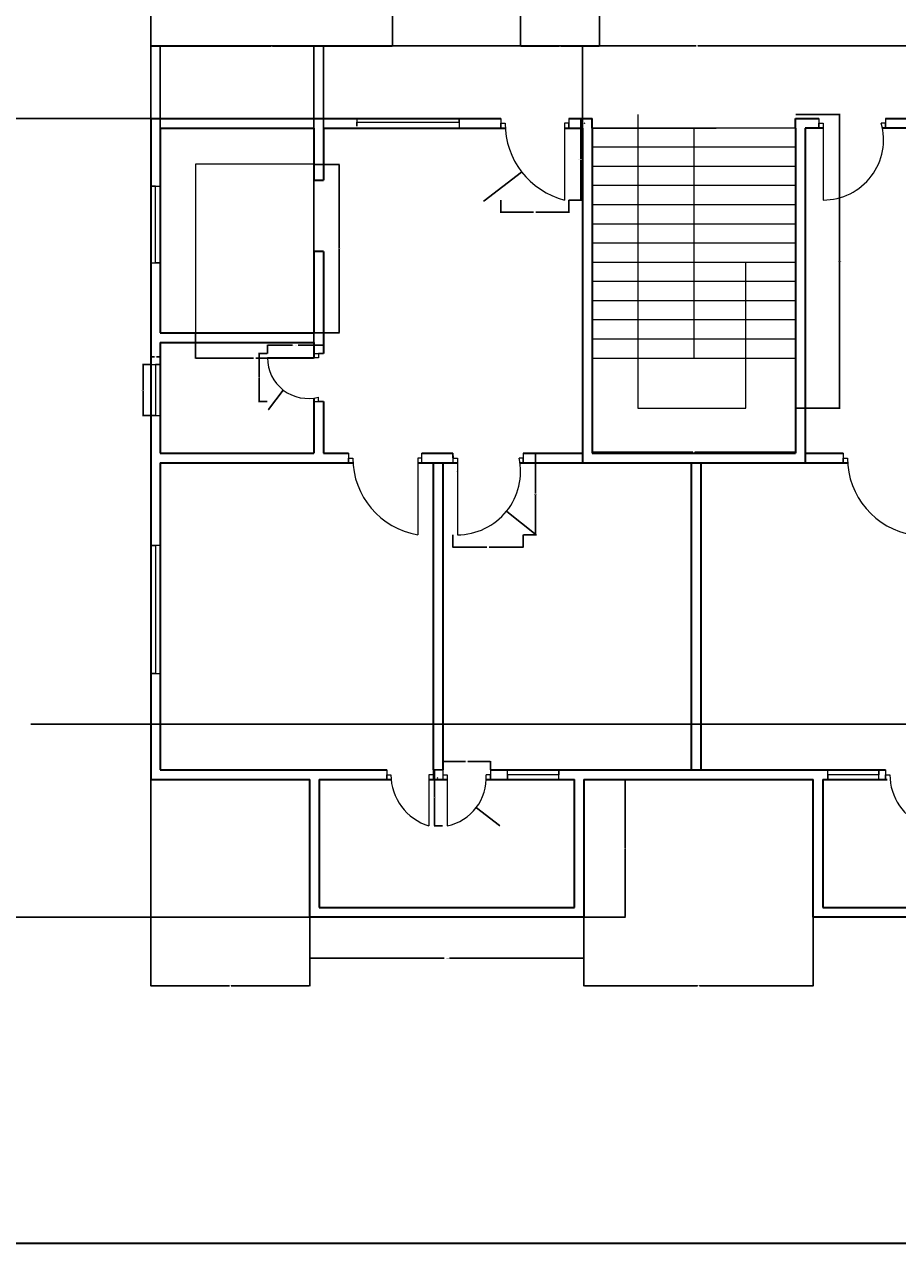
# Model space of a CAD drawing. Units: inches. Extents: x 2055 to 3558, y 1520 to 2888.
# Tile 5 of 8: x 2732 to 3142, y 1520 to 2092. Entities that reach past the tile are written whole.
import ezdxf

# ---------------------------------------------------------------- set-up
doc = ezdxf.new("R2010")
doc.units = ezdxf.units.IN
for name, color, linetype, lineweight in [('A-ANNO-DIMS', 2, 'Continuous', 18), ('A-ANNO-SYMB', 7, 'Continuous', 25), ('A-ANNO-TTLB', 7, 'Continuous', 35), ('A-DOOR', 3, 'Continuous', 18), ('A-FLOR-FIXT', 8, 'Continuous', 18), ('A-FLOR-STRS', 7, 'Continuous', 18), ('A-GLAZ', 4, 'Continuous', 18), ('A-WALL', 7, 'Continuous', 35)]:
    doc.layers.add(name, color=color, linetype=linetype, lineweight=lineweight)
doc.styles.get("Standard").update_dxf_attribs({"font": 'arial.ttf'})
doc.dimstyles.get("Standard").update_dxf_attribs({"dimtxt": 0.18, "dimasz": 0.18, "dimexe": 0.18, "dimexo": 0.0625, "dimgap": 0.09, "dimtad": 0, "dimtih": 1, "dimtoh": 1, "dimdec": 4, "dimzin": 0, "dimdsep": 46, "dimtxsty": 'Standard', "dimcen": 0.09, "dimadec": 0, "dimazin": 0, "dimtfac": 1, "dimtdec": 4, "dimtofl": 0, "dimtmove": 0, "dimatfit": 3, "dimfxl": 1, "dimtolj": 1, "dimtzin": 0, "dimarcsym": 0})

# ---------------------------------------------------------------- blocks, each defined once
blk = doc.blocks.new('DOOR-ENTRY-36-C')
for p, q in [((0, 38.25), (0, 33.75)), ((0, 33.75), (0, 36)), ((0, 36), (2, 36)), ((31.88, 36), (29.88, 36)), ((29.88, 36), (29.88, 0)), ((31.88, 38.25), (31.88, 33.75)), ((31.88, 33.75), (31.88, 36))]:
    blk.add_line(p, q)
blk.add_arc((39.18, 36), 37.18, 180, 255.5126)
blk = doc.blocks.new('DOOR-BATH-24-C')
for p, q in [((24, 20.46), (0, 20.46)), ((21.75, 22.46), (26.25, 22.46)), ((26.25, 22.46), (24, 22.46)), ((24, 22.46), (24, 20.46)), ((24, 0), (24, 2)), ((21.75, 0), (26.25, 0)), ((26.25, 0), (24, 0))]:
    blk.add_line(p, q)
blk.add_arc((19.1, 20.46), 19.1, 180, 284.8648)
blk = doc.blocks.new('DOOR-ENTRY-36-D')
for p, q in [((0, 38.25), (0, 33.75)), ((0, 33.75), (0, 36)), ((0, 36), (2, 36)), ((2, 36), (2, 0)), ((31.26, 36), (29.26, 36)), ((31.26, 38.25), (31.26, 33.75)), ((31.26, 33.75), (31.26, 36))]:
    blk.add_line(p, q)
blk.add_arc((2, 28.32), 28.32, 270, 15.7411)
blk = doc.blocks.new('DOOR-BED-36-D')
for p, q in [((0.16, 33.75), (0, 38.25)), ((0, 38.25), (0.08, 36)), ((0.08, 36), (2.08, 36)), ((2.08, 36), (2.08, 0)), ((33, 36), (31, 36)), ((33, 38.25), (33, 33.75)), ((33, 33.75), (33, 36))]:
    blk.add_line(p, q)
blk.add_arc((2.08, 29.62), 29.61, 270, 12.4519)
blk = doc.blocks.new('DOOR-BED-36-E')
for p, q in [((0, 38.25), (0, 33.75)), ((0, 33.75), (0, 36)), ((0, 36), (2, 36)), ((34.42, 36), (32.42, 36)), ((32.42, 36), (32.42, 0)), ((34.42, 33.75), (34.42, 38.25))]:
    blk.add_line(p, q)
blk.add_arc((38.51, 36), 36.51, 180, 260.3872)
blk = doc.blocks.new('DOOR-BED-36-G')
for p, q in [((0, 38.25), (0, 33.75)), ((0, 33.75), (0, 36)), ((0, 36), (2, 36)), ((34.89, 36), (32.89, 36)), ((32.89, 36), (32.89, 0)), ((34.89, 38.25), (34.89, 33.75)), ((34.89, 33.75), (34.89, 36))]:
    blk.add_line(p, q)
blk.add_arc((38.42, 36), 36.42, 180, 261.253)
blk = doc.blocks.new('DOOR-VERANDA-24-B')
for p, q in [((0, 26.25), (0, 21.75)), ((0, 21.75), (0, 24)), ((0, 24), (2, 24)), ((20.42, 24), (18.42, 24)), ((18.42, 24), (18.42, 0)), ((20.42, 26.25), (20.42, 21.75))]:
    blk.add_line(p, q)
blk.add_arc((27.75, 24), 25.75, 180, 248.7547)
blk = doc.blocks.new('DOOR-VERANDA-24-C')
for p, q in [((0, 26.25), (0, 21.75)), ((0, 21.75), (0, 24)), ((0, 24), (2, 24)), ((21.82, 24), (19.82, 24)), ((19.82, 24), (19.82, 0)), ((21.82, 26.25), (21.82, 21.75))]:
    blk.add_line(p, q)
blk.add_arc((27.07, 24), 25.07, 180, 253.1988)
blk = doc.blocks.new('DOOR-VERANDA-24-D')
for p, q in [((0, 26.25), (0, 21.75)), ((0, 24), (2, 24)), ((2, 24), (2, 0)), ((22.33, 24), (20.33, 24)), ((22.33, 26.25), (22.33, 21.75)), ((22.33, 21.75), (22.33, 24))]:
    blk.add_line(p, q)
blk.add_arc((-2.55, 22.48), 22.94, 281.4505, 3.8037)
blk = doc.blocks.new('WIN-36')
for p, q in [((2.25, 36), (0, 36)), ((0, 36), (4.5, 36)), ((2.25, 0), (2.25, 36)), ((0, 0), (4.5, 0)), ((4.5, 0), (2.25, 0))]:
    blk.add_line(p, q)
blk = doc.blocks.new('WIN-24')
for p, q in [((0, 24), (4.5, 24)), ((4.5, 24), (2.25, 24)), ((2.25, 24), (2.25, 0)), ((2.25, 0), (0, 0)), ((0, 0), (4.5, 0))]:
    blk.add_line(p, q)
blk = doc.blocks.new('WIN-60-2')
for p, q in [((4.5, 60), (0, 60)), ((0, 60), (2.25, 60)), ((2.25, 60), (2.25, 0)), ((2.25, 0), (0, 0)), ((0, 0), (4.5, 0))]:
    blk.add_line(p, q)
blk = doc.blocks.new('WIN-48-2')
for p, q in [((0, 4.5), (0, 0.97)), ((0, 0.97), (0, 2.74)), ((0, 2.74), (48, 2.74)), ((48, 2.74), (48, 4.5)), ((48, 4.5), (48, 0))]:
    blk.add_line(p, q)
blk = doc.blocks.new('COUNTER-3')
for p, q in [((55.49, 79.01), (0, 79.01)), ((0, 79.01), (0, 0))]:
    blk.add_line(p, q)
blk = doc.blocks.new('VERANDA-PERIMETER')
for p, q in [((0, 0), (0, 64.5)), ((4.5, 64.5), (4.5, 4.5)), ((124.15, 4.5), (124.15, 64.5)), ((128.65, 64.5), (128.65, 4.5)), ((4.5, 0), (0, 0)), ((4.5, 4.5), (124.15, 4.5)), ((128.65, 0), (4.5, 0)), ((128.65, 4.5), (128.65, 0))]:
    blk.add_line(p, q)
blk = doc.blocks.new('STAIR-RETURN')
for p, q in [((21.46, 137.78), (21.46, 0)), ((95.44, 131.38), (0, 131.38)), ((0, 131.38), (58.19, 131.38)), ((47.72, 131.38), (47.72, 23.38)), ((95.44, 122.38), (0, 122.38)), ((95.44, 113.38), (0, 113.38)), ((95.44, 104.38), (0, 104.38)), ((95.44, 95.38), (0, 95.38)), ((95.44, 86.38), (0, 86.38)), ((95.44, 77.38), (0, 77.38)), ((95.44, 68.38), (0, 68.38)), ((72.2, 0), (72.2, 68.38)), ((95.44, 59.38), (0, 59.38)), ((95.44, 50.38), (0, 50.38)), ((95.44, 41.38), (0, 41.38)), ((95.44, 32.38), (0, 32.38)), ((95.44, 23.38), (0, 23.38)), ((21.46, 0), (72.2, 0))]:
    blk.add_line(p, q)
blk = doc.blocks.new('*D40')
at = {"layer": 'A-ANNO-DIMS', "color": 0, "lineweight": -2, "transparency": 16777216}
for p, q in [((2791.43, 1932.63), (2787.72, 1932.63)), ((2787.9, 1932.45), (2787.9, 1920.81)), ((2787.9, 1908.81), (2787.9, 1920.45)), ((2791.43, 1908.63), (2787.72, 1908.63))]:
    blk.add_line(p, q, dxfattribs=at)
at = {"layer": 'A-ANNO-DIMS', "color": 0, "transparency": 16777216}
for points in [[(2787.87, 1932.45), (2787.93, 1932.45), (2787.9, 1932.63)], [(2787.87, 1908.81), (2787.93, 1908.81), (2787.9, 1908.63)]]:
    blk.add_solid(points, dxfattribs=at)
at = {"layer": 'Defpoints', "color": 0, "transparency": 16777216}
for p in [(2787.9, 1932.63), (2791.5, 1932.63), (2791.5, 1908.63)]:
    blk.add_point(p, dxfattribs=at)
at = {"layer": 'A-ANNO-DIMS', "color": 0, "transparency": 16777216, "insert": (2787.9, 1920.63), "char_height": 0.18, "attachment_point": 5}
blk.add_mtext('\\A1;WINDOW 24 TYP.', dxfattribs=at)
blk = doc.blocks.new('*D41')
at = {"layer": 'A-ANNO-DIMS', "color": 0, "lineweight": -2, "transparency": 16777216}
for p, q in [((2791.5, 1932.69), (2791.5, 1936.41)), ((2791.68, 1936.23), (2793.29, 1936.23)), ((2795.82, 1936.23), (2794.2, 1936.23)), ((2796, 1932.69), (2796, 1936.41))]:
    blk.add_line(p, q, dxfattribs=at)
at = {"layer": 'A-ANNO-DIMS', "color": 0, "transparency": 16777216}
for points in [[(2791.68, 1936.26), (2791.68, 1936.2), (2791.5, 1936.23)], [(2795.82, 1936.26), (2795.82, 1936.2), (2796, 1936.23)]]:
    blk.add_solid(points, dxfattribs=at)
at = {"layer": 'Defpoints', "color": 0, "transparency": 16777216}
for p in [(2796, 1936.23), (2791.5, 1932.63), (2796, 1932.63)]:
    blk.add_point(p, dxfattribs=at)
at = {"layer": 'A-ANNO-DIMS', "color": 0, "transparency": 16777216, "insert": (2793.75, 1936.23), "char_height": 0.18, "attachment_point": 5}
blk.add_mtext('\\A1;5 TYP.', dxfattribs=at)
blk = doc.blocks.new('*D46')
at = {"layer": 'A-ANNO-DIMS', "color": 0, "lineweight": -2, "transparency": 16777216}
for p, q in [((2866.07, 1673.44), (2866.07, 1654.02)), ((2994.71, 1673.44), (2994.71, 1654.02)), ((2866.25, 1654.2), (2929.14, 1654.2)), ((2994.53, 1654.2), (2931.63, 1654.2))]:
    blk.add_line(p, q, dxfattribs=at)
at = {"layer": 'A-ANNO-DIMS', "color": 0, "transparency": 16777216}
for points in [[(2866.25, 1654.23), (2866.25, 1654.17), (2866.07, 1654.2)], [(2994.53, 1654.23), (2994.53, 1654.17), (2994.71, 1654.2)]]:
    blk.add_solid(points, dxfattribs=at)
at = {"layer": 'Defpoints', "color": 0, "transparency": 16777216}
for p in [(2866.07, 1673.5), (2994.71, 1673.5), (2994.71, 1654.2)]:
    blk.add_point(p, dxfattribs=at)
at = {"layer": 'A-ANNO-DIMS', "color": 0, "transparency": 16777216, "insert": (2930.39, 1654.2), "char_height": 0.18, "attachment_point": 5}
blk.add_mtext('\\A1;VERANDA 129 TYP.', dxfattribs=at)
blk = doc.blocks.new('*D47')
at = {"layer": 'A-ANNO-DIMS', "color": 0, "lineweight": -2, "transparency": 16777216}
for p, q in [((2994.77, 1738), (3014.19, 1738)), ((3014.01, 1737.82), (3014.01, 1705.93)), ((3014.01, 1673.68), (3014.01, 1705.57)), ((2994.77, 1673.5), (3014.19, 1673.5))]:
    blk.add_line(p, q, dxfattribs=at)
at = {"layer": 'A-ANNO-DIMS', "color": 0, "transparency": 16777216}
for points in [[(3013.98, 1737.82), (3014.04, 1737.82), (3014.01, 1738)], [(3013.98, 1673.68), (3014.04, 1673.68), (3014.01, 1673.5)]]:
    blk.add_solid(points, dxfattribs=at)
at = {"layer": 'Defpoints', "color": 0, "transparency": 16777216}
for p in [(2994.71, 1738), (3014.01, 1738), (2994.71, 1673.5)]:
    blk.add_point(p, dxfattribs=at)
at = {"layer": 'A-ANNO-DIMS', "color": 0, "transparency": 16777216, "insert": (3014.01, 1705.75), "char_height": 0.18, "attachment_point": 5}
blk.add_mtext('\\A1;65 TYP.', dxfattribs=at)
blk = doc.blocks.new('*D66')
at = {"layer": 'A-ANNO-DIMS', "color": 0, "lineweight": -2, "transparency": 16777216}
for p, q in [((2987.64, 2048), (2993.49, 2048)), ((2993.31, 2047.82), (2993.31, 2029.06)), ((2993.31, 2009.93), (2993.31, 2028.69)), ((2987.64, 2009.75), (2993.49, 2009.75))]:
    blk.add_line(p, q, dxfattribs=at)
at = {"layer": 'A-ANNO-DIMS', "color": 0, "transparency": 16777216}
for points in [[(2993.28, 2047.82), (2993.34, 2047.82), (2993.31, 2048)], [(2993.28, 2009.93), (2993.34, 2009.93), (2993.31, 2009.75)]]:
    blk.add_solid(points, dxfattribs=at)
at = {"layer": 'Defpoints', "color": 0, "transparency": 16777216}
for p in [(2987.58, 2048), (2993.31, 2048), (2987.58, 2009.75)]:
    blk.add_point(p, dxfattribs=at)
at = {"layer": 'A-ANNO-DIMS', "color": 0, "transparency": 16777216, "insert": (2993.31, 2028.87), "char_height": 0.18, "attachment_point": 5}
blk.add_mtext('\\A1;ENTRY DOOR 38 TYP.', dxfattribs=at)
blk = doc.blocks.new('*D67')
at = {"layer": 'A-ANNO-DIMS', "color": 0, "lineweight": -2, "transparency": 16777216}
for p, q in [((2955.7, 2009.69), (2955.7, 2003.83)), ((2987.58, 2009.69), (2987.58, 2003.83)), ((2955.88, 2004.01), (2971.11, 2004.01)), ((2987.4, 2004.01), (2972.16, 2004.01))]:
    blk.add_line(p, q, dxfattribs=at)
at = {"layer": 'A-ANNO-DIMS', "color": 0, "transparency": 16777216}
for points in [[(2955.88, 2004.04), (2955.88, 2003.98), (2955.7, 2004.01)], [(2987.4, 2004.04), (2987.4, 2003.98), (2987.58, 2004.01)]]:
    blk.add_solid(points, dxfattribs=at)
at = {"layer": 'Defpoints', "color": 0, "transparency": 16777216}
for p in [(2955.7, 2009.75), (2987.58, 2009.75), (2987.58, 2004.01)]:
    blk.add_point(p, dxfattribs=at)
at = {"layer": 'A-ANNO-DIMS', "color": 0, "transparency": 16777216, "insert": (2971.64, 2004.01), "char_height": 0.18, "attachment_point": 5}
blk.add_mtext('\\A1;32 TYP.', dxfattribs=at)
blk = doc.blocks.new('*D70')
at = {"layer": 'A-ANNO-DIMS', "color": 0, "lineweight": -2, "transparency": 16777216}
for p, q in [((2846.25, 1937.85), (2846.25, 1941.91)), ((2846.43, 1941.73), (2858.06, 1941.73)), ((2872.32, 1941.73), (2860.68, 1941.73)), ((2872.5, 1937.85), (2872.5, 1941.91))]:
    blk.add_line(p, q, dxfattribs=at)
at = {"layer": 'A-ANNO-DIMS', "color": 0, "transparency": 16777216}
for points in [[(2846.43, 1941.76), (2846.43, 1941.7), (2846.25, 1941.73)], [(2872.32, 1941.76), (2872.32, 1941.7), (2872.5, 1941.73)]]:
    blk.add_solid(points, dxfattribs=at)
at = {"layer": 'Defpoints', "color": 0, "transparency": 16777216}
for p in [(2872.5, 1941.73), (2846.25, 1937.79), (2872.5, 1937.79)]:
    blk.add_point(p, dxfattribs=at)
at = {"layer": 'A-ANNO-DIMS', "color": 0, "transparency": 16777216, "insert": (2859.37, 1941.73), "char_height": 0.18, "attachment_point": 5}
blk.add_mtext('\\A1;BATH DOOR 26 TYP.', dxfattribs=at)
blk = doc.blocks.new('*D71')
at = {"layer": 'A-ANNO-DIMS', "color": 0, "lineweight": -2, "transparency": 16777216}
for p, q in [((2846.18, 1937.79), (2842.13, 1937.79)), ((2842.31, 1937.61), (2842.31, 1926.74)), ((2842.31, 1915.51), (2842.31, 1926.38)), ((2846.18, 1915.33), (2842.13, 1915.33))]:
    blk.add_line(p, q, dxfattribs=at)
at = {"layer": 'A-ANNO-DIMS', "color": 0, "transparency": 16777216}
for points in [[(2842.28, 1937.61), (2842.34, 1937.61), (2842.31, 1937.79)], [(2842.28, 1915.51), (2842.34, 1915.51), (2842.31, 1915.33)]]:
    blk.add_solid(points, dxfattribs=at)
at = {"layer": 'Defpoints', "color": 0, "transparency": 16777216}
for p in [(2842.31, 1937.79), (2846.25, 1937.79), (2846.25, 1915.33)]:
    blk.add_point(p, dxfattribs=at)
at = {"layer": 'A-ANNO-DIMS', "color": 0, "transparency": 16777216, "insert": (2842.31, 1926.56), "char_height": 0.18, "attachment_point": 5}
blk.add_mtext('\\A1;22 TYP.', dxfattribs=at)
blk = doc.blocks.new('*D74')
at = {"layer": 'A-ANNO-DIMS', "color": 0, "lineweight": -2, "transparency": 16777216}
for p, q in [((2966.31, 1891), (2972.16, 1891)), ((2971.98, 1890.82), (2971.98, 1872.06)), ((2971.98, 1852.93), (2971.98, 1871.69)), ((2966.31, 1852.75), (2972.16, 1852.75))]:
    blk.add_line(p, q, dxfattribs=at)
at = {"layer": 'A-ANNO-DIMS', "color": 0, "transparency": 16777216}
for points in [[(2971.95, 1890.82), (2972.01, 1890.82), (2971.98, 1891)], [(2971.95, 1852.93), (2972.01, 1852.93), (2971.98, 1852.75)]]:
    blk.add_solid(points, dxfattribs=at)
at = {"layer": 'Defpoints', "color": 0, "transparency": 16777216}
for p in [(2966.24, 1891), (2971.98, 1891), (2966.24, 1852.75)]:
    blk.add_point(p, dxfattribs=at)
at = {"layer": 'A-ANNO-DIMS', "color": 0, "transparency": 16777216, "insert": (2971.98, 1871.87), "char_height": 0.18, "attachment_point": 5}
blk.add_mtext('\\A1;BED DOOR 38 TYP.', dxfattribs=at)
blk = doc.blocks.new('*D75')
at = {"layer": 'A-ANNO-DIMS', "color": 0, "lineweight": -2, "transparency": 16777216}
for p, q in [((2933.25, 1852.69), (2933.25, 1846.83)), ((2966.24, 1852.69), (2966.24, 1846.83)), ((2933.43, 1847.01), (2949.22, 1847.01)), ((2966.06, 1847.01), (2950.27, 1847.01))]:
    blk.add_line(p, q, dxfattribs=at)
at = {"layer": 'A-ANNO-DIMS', "color": 0, "transparency": 16777216}
for points in [[(2933.43, 1847.04), (2933.43, 1846.98), (2933.25, 1847.01)], [(2966.06, 1847.04), (2966.06, 1846.98), (2966.24, 1847.01)]]:
    blk.add_solid(points, dxfattribs=at)
at = {"layer": 'Defpoints', "color": 0, "transparency": 16777216}
for p in [(2933.25, 1852.75), (2966.24, 1852.75), (2966.24, 1847.01)]:
    blk.add_point(p, dxfattribs=at)
at = {"layer": 'A-ANNO-DIMS', "color": 0, "transparency": 16777216, "insert": (2949.74, 1847.01), "char_height": 0.18, "attachment_point": 5}
blk.add_mtext('\\A1;33 TYP.', dxfattribs=at)
blk = doc.blocks.new('*D88')
at = {"layer": 'A-ANNO-DIMS', "color": 0, "lineweight": -2, "transparency": 16777216}
for p, q in [((2928.43, 1742.5), (2924.38, 1742.5)), ((2924.56, 1742.32), (2924.56, 1729.56)), ((2924.56, 1716.43), (2924.56, 1729.19)), ((2928.43, 1716.25), (2924.38, 1716.25))]:
    blk.add_line(p, q, dxfattribs=at)
at = {"layer": 'A-ANNO-DIMS', "color": 0, "transparency": 16777216}
for points in [[(2924.53, 1742.32), (2924.59, 1742.32), (2924.56, 1742.5)], [(2924.53, 1716.43), (2924.59, 1716.43), (2924.56, 1716.25)]]:
    blk.add_solid(points, dxfattribs=at)
at = {"layer": 'Defpoints', "color": 0, "transparency": 16777216}
for p in [(2924.56, 1742.5), (2928.5, 1742.5), (2928.5, 1716.25)]:
    blk.add_point(p, dxfattribs=at)
at = {"layer": 'A-ANNO-DIMS', "color": 0, "transparency": 16777216, "insert": (2924.56, 1729.37), "char_height": 0.18, "attachment_point": 5}
blk.add_mtext('\\A1;DOOR 26 TYP.', dxfattribs=at)
blk = doc.blocks.new('*D89')
at = {"layer": 'A-ANNO-DIMS', "color": 0, "lineweight": -2, "transparency": 16777216}
for p, q in [((2928.5, 1742.56), (2928.5, 1746.62)), ((2928.68, 1746.44), (2939.13, 1746.44)), ((2950.65, 1746.44), (2940.19, 1746.44)), ((2950.83, 1742.56), (2950.83, 1746.62))]:
    blk.add_line(p, q, dxfattribs=at)
at = {"layer": 'A-ANNO-DIMS', "color": 0, "transparency": 16777216}
for points in [[(2928.68, 1746.47), (2928.68, 1746.41), (2928.5, 1746.44)], [(2950.65, 1746.47), (2950.65, 1746.41), (2950.83, 1746.44)]]:
    blk.add_solid(points, dxfattribs=at)
at = {"layer": 'Defpoints', "color": 0, "transparency": 16777216}
for p in [(2950.83, 1746.44), (2928.5, 1742.5), (2950.83, 1742.5)]:
    blk.add_point(p, dxfattribs=at)
at = {"layer": 'A-ANNO-DIMS', "color": 0, "transparency": 16777216, "insert": (2939.66, 1746.44), "char_height": 0.18, "attachment_point": 5}
blk.add_mtext('\\A1;22 TYP.', dxfattribs=at)
blk = doc.blocks.new('*D110')
at = {"layer": 'A-ANNO-DIMS', "color": 0, "lineweight": -2, "transparency": 16777216}
for p, q in [((2868.06, 2026.5), (2880.03, 2026.5)), ((2879.85, 2026.32), (2879.85, 1987.19)), ((2879.85, 1947.68), (2879.85, 1986.82)), ((2868.06, 1947.5), (2880.03, 1947.5))]:
    blk.add_line(p, q, dxfattribs=at)
at = {"layer": 'A-ANNO-DIMS', "color": 0, "transparency": 16777216}
for points in [[(2879.82, 2026.32), (2879.88, 2026.32), (2879.85, 2026.5)], [(2879.82, 1947.68), (2879.88, 1947.68), (2879.85, 1947.5)]]:
    blk.add_solid(points, dxfattribs=at)
at = {"layer": 'Defpoints', "color": 0, "transparency": 16777216}
for p in [(2868, 2026.5), (2879.85, 2026.5), (2868, 1947.5)]:
    blk.add_point(p, dxfattribs=at)
at = {"layer": 'A-ANNO-DIMS', "color": 0, "transparency": 16777216, "insert": (2879.85, 1987), "char_height": 0.18, "attachment_point": 5}
blk.add_mtext('\\A1;COUNTER 79 TYP.', dxfattribs=at)
blk = doc.blocks.new('*D111')
at = {"layer": 'A-ANNO-DIMS', "color": 0, "lineweight": -2, "transparency": 16777216}
for p, q in [((2812.51, 1947.44), (2812.51, 1935.47)), ((2868, 1947.44), (2868, 1935.47)), ((2812.69, 1935.65), (2839.72, 1935.65)), ((2867.82, 1935.65), (2840.78, 1935.65))]:
    blk.add_line(p, q, dxfattribs=at)
at = {"layer": 'A-ANNO-DIMS', "color": 0, "transparency": 16777216}
for points in [[(2812.69, 1935.68), (2812.69, 1935.62), (2812.51, 1935.65)], [(2867.82, 1935.68), (2867.82, 1935.62), (2868, 1935.65)]]:
    blk.add_solid(points, dxfattribs=at)
at = {"layer": 'Defpoints', "color": 0, "transparency": 16777216}
for p in [(2812.51, 1947.5), (2868, 1947.5), (2868, 1935.65)]:
    blk.add_point(p, dxfattribs=at)
at = {"layer": 'A-ANNO-DIMS', "color": 0, "transparency": 16777216, "insert": (2840.25, 1935.65), "char_height": 0.18, "attachment_point": 5}
blk.add_mtext('\\A1;55 TYP.', dxfattribs=at)
blk = doc.blocks.new('*D114')
at = {"layer": 'A-ANNO-DIMS', "color": 0, "lineweight": -2, "transparency": 16777216}
for p, q in [((3094, 2049.9), (3114.79, 2049.9)), ((3114.61, 2049.72), (3114.61, 1981.19)), ((3114.61, 1912.3), (3114.61, 1980.83)), ((3094, 1912.12), (3114.79, 1912.12))]:
    blk.add_line(p, q, dxfattribs=at)
at = {"layer": 'A-ANNO-DIMS', "color": 0, "transparency": 16777216}
for points in [[(3114.58, 2049.72), (3114.64, 2049.72), (3114.61, 2049.9)], [(3114.58, 1912.3), (3114.64, 1912.3), (3114.61, 1912.12)]]:
    blk.add_solid(points, dxfattribs=at)
at = {"layer": 'Defpoints', "color": 0, "transparency": 16777216}
for p in [(3093.94, 2049.9), (3114.61, 2049.9), (3093.94, 1912.12)]:
    blk.add_point(p, dxfattribs=at)
at = {"layer": 'A-ANNO-DIMS', "color": 0, "transparency": 16777216, "insert": (3114.61, 1981.01), "char_height": 0.18, "attachment_point": 5}
blk.add_mtext('\\A1;STAIR 138 TYP.', dxfattribs=at)
blk = doc.blocks.new('*D115')
at = {"layer": 'A-ANNO-DIMS', "color": 0, "lineweight": -2, "transparency": 16777216}
for p, q in [((2998.5, 1912.06), (2998.5, 1891.27)), ((3093.94, 1912.06), (3093.94, 1891.27)), ((2998.68, 1891.45), (3045.69, 1891.45)), ((3093.76, 1891.45), (3046.75, 1891.45))]:
    blk.add_line(p, q, dxfattribs=at)
at = {"layer": 'A-ANNO-DIMS', "color": 0, "transparency": 16777216}
for points in [[(2998.68, 1891.48), (2998.68, 1891.42), (2998.5, 1891.45)], [(3093.76, 1891.48), (3093.76, 1891.42), (3093.94, 1891.45)]]:
    blk.add_solid(points, dxfattribs=at)
at = {"layer": 'Defpoints', "color": 0, "transparency": 16777216}
for p in [(2998.5, 1912.12), (3093.94, 1912.12), (3093.94, 1891.45)]:
    blk.add_point(p, dxfattribs=at)
at = {"layer": 'A-ANNO-DIMS', "color": 0, "transparency": 16777216, "insert": (3046.22, 1891.45), "char_height": 0.18, "attachment_point": 5}
blk.add_mtext('\\A1;95 TYP.', dxfattribs=at)
blk = doc.blocks.new('*D128')
at = {"layer": 'A-ANNO-DIMS', "color": 0, "lineweight": -2, "transparency": 16777216}
for p, q in [((2791.5, 2107.94), (2791.5, 2081.72)), ((2904.9, 2107.94), (2904.9, 2081.72)), ((2791.68, 2081.9), (2847.81, 2081.9)), ((2904.72, 2081.9), (2848.58, 2081.9))]:
    blk.add_line(p, q, dxfattribs=at)
at = {"layer": 'A-ANNO-DIMS', "color": 0, "transparency": 16777216}
for points in [[(2791.68, 2081.93), (2791.68, 2081.87), (2791.5, 2081.9)], [(2904.72, 2081.93), (2904.72, 2081.87), (2904.9, 2081.9)]]:
    blk.add_solid(points, dxfattribs=at)
at = {"layer": 'Defpoints', "color": 0, "transparency": 16777216}
for p in [(2791.5, 2108), (2904.9, 2108), (2904.9, 2081.9)]:
    blk.add_point(p, dxfattribs=at)
at = {"layer": 'A-ANNO-DIMS', "color": 0, "transparency": 16777216, "insert": (2848.2, 2081.9), "char_height": 0.18, "attachment_point": 5}
blk.add_mtext('\\A1;113.4', dxfattribs=at)
blk = doc.blocks.new('*D129')
at = {"layer": 'A-ANNO-DIMS', "color": 0, "lineweight": -2, "transparency": 16777216}
for p, q in [((2964.9, 2107.94), (2964.9, 2081.72)), ((3001.98, 2107.94), (3001.98, 2081.72)), ((2965.08, 2081.9), (2983.05, 2081.9)), ((3001.8, 2081.9), (2983.83, 2081.9))]:
    blk.add_line(p, q, dxfattribs=at)
at = {"layer": 'A-ANNO-DIMS', "color": 0, "transparency": 16777216}
for points in [[(2965.08, 2081.93), (2965.08, 2081.87), (2964.9, 2081.9)], [(3001.8, 2081.93), (3001.8, 2081.87), (3001.98, 2081.9)]]:
    blk.add_solid(points, dxfattribs=at)
at = {"layer": 'Defpoints', "color": 0, "transparency": 16777216}
for p in [(2964.9, 2108), (3001.98, 2108), (3001.98, 2081.9)]:
    blk.add_point(p, dxfattribs=at)
at = {"layer": 'A-ANNO-DIMS', "color": 0, "transparency": 16777216, "insert": (2983.44, 2081.9), "char_height": 0.18, "attachment_point": 5}
blk.add_mtext('\\A1;37.08', dxfattribs=at)
blk = doc.blocks.new('*D133')
at = {"layer": 'A-ANNO-DIMS', "color": 0, "lineweight": -2, "transparency": 16777216}
for p, q in [((2791.5, 2048.06), (2791.5, 2082.28)), ((2791.68, 2082.1), (3047.35, 2082.1)), ((3303.82, 2082.1), (3048.14, 2082.1)), ((3304, 2048.06), (3304, 2082.28))]:
    blk.add_line(p, q, dxfattribs=at)
at = {"layer": 'A-ANNO-DIMS', "color": 0, "transparency": 16777216}
for points in [[(2791.68, 2082.13), (2791.68, 2082.07), (2791.5, 2082.1)], [(3303.82, 2082.13), (3303.82, 2082.07), (3304, 2082.1)]]:
    blk.add_solid(points, dxfattribs=at)
at = {"layer": 'Defpoints', "color": 0, "transparency": 16777216}
for p in [(3304, 2082.1), (2791.5, 2048), (3304, 2048)]:
    blk.add_point(p, dxfattribs=at)
at = {"layer": 'A-ANNO-DIMS', "color": 0, "transparency": 16777216, "insert": (3047.75, 2082.1), "char_height": 0.18, "attachment_point": 5}
blk.add_mtext('\\A1;512.5', dxfattribs=at)
blk = doc.blocks.new('*D134')
at = {"layer": 'A-ANNO-DIMS', "color": 0, "lineweight": -2, "transparency": 16777216}
for p, q in [((2791.43, 2048), (2702.83, 2048)), ((2703.01, 2047.82), (2703.01, 1860.93)), ((2703.01, 1673.68), (2703.01, 1860.57)), ((2866, 1673.5), (2702.83, 1673.5))]:
    blk.add_line(p, q, dxfattribs=at)
at = {"layer": 'A-ANNO-DIMS', "color": 0, "transparency": 16777216}
for points in [[(2702.98, 2047.82), (2703.04, 2047.82), (2703.01, 2048)], [(2702.98, 1673.68), (2703.04, 1673.68), (2703.01, 1673.5)]]:
    blk.add_solid(points, dxfattribs=at)
at = {"layer": 'Defpoints', "color": 0, "transparency": 16777216}
for p in [(2791.5, 2048), (2703.01, 1673.5), (2866.07, 1673.5)]:
    blk.add_point(p, dxfattribs=at)
at = {"layer": 'A-ANNO-DIMS', "color": 0, "transparency": 16777216, "insert": (2703.01, 1860.75), "char_height": 0.18, "attachment_point": 5}
blk.add_mtext('\\A1;374.5', dxfattribs=at)
blk = doc.blocks.new('*D135')
at = {"layer": 'A-ANNO-DIMS', "color": 0, "lineweight": -2, "transparency": 16777216}
for p, q in [((2791.5, 1737.94), (2791.5, 1641.12)), ((2866.07, 1737.94), (2866.07, 1641.12)), ((2791.68, 1641.3), (2828.39, 1641.3)), ((2865.89, 1641.3), (2829.17, 1641.3))]:
    blk.add_line(p, q, dxfattribs=at)
at = {"layer": 'A-ANNO-DIMS', "color": 0, "transparency": 16777216}
for points in [[(2791.68, 1641.33), (2791.68, 1641.27), (2791.5, 1641.3)], [(2865.89, 1641.33), (2865.89, 1641.27), (2866.07, 1641.3)]]:
    blk.add_solid(points, dxfattribs=at)
at = {"layer": 'Defpoints', "color": 0, "transparency": 16777216}
for p in [(2791.5, 1738), (2866.07, 1738), (2866.07, 1641.3)]:
    blk.add_point(p, dxfattribs=at)
at = {"layer": 'A-ANNO-DIMS', "color": 0, "transparency": 16777216, "insert": (2828.78, 1641.3), "char_height": 0.18, "attachment_point": 5}
blk.add_mtext('\\A1;74.57', dxfattribs=at)
blk = doc.blocks.new('*D136')
at = {"layer": 'A-ANNO-DIMS', "color": 0, "lineweight": -2, "transparency": 16777216}
for p, q in [((2994.71, 1673.44), (2994.71, 1641.12)), ((3102.17, 1673.44), (3102.17, 1641.12)), ((2994.89, 1641.3), (3047.98, 1641.3)), ((3101.99, 1641.3), (3048.89, 1641.3))]:
    blk.add_line(p, q, dxfattribs=at)
at = {"layer": 'A-ANNO-DIMS', "color": 0, "transparency": 16777216}
for points in [[(2994.89, 1641.33), (2994.89, 1641.27), (2994.71, 1641.3)], [(3101.99, 1641.33), (3101.99, 1641.27), (3102.17, 1641.3)]]:
    blk.add_solid(points, dxfattribs=at)
at = {"layer": 'Defpoints', "color": 0, "transparency": 16777216}
for p in [(2994.71, 1673.5), (3102.17, 1673.5), (3102.17, 1641.3)]:
    blk.add_point(p, dxfattribs=at)
at = {"layer": 'A-ANNO-DIMS', "color": 0, "transparency": 16777216, "insert": (3048.44, 1641.3), "char_height": 0.18, "attachment_point": 5}
blk.add_mtext('\\A1;107.45', dxfattribs=at)
blk = doc.blocks.new('*D137')
at = {"layer": 'A-ANNO-DIMS', "color": 0, "lineweight": -2, "transparency": 16777216}
for p, q in [((2796, 1947.56), (2796, 2082.28)), ((2796.18, 2082.1), (2831.78, 2082.1)), ((2867.82, 2082.1), (2832.21, 2082.1)), ((2868, 1947.56), (2868, 2082.28))]:
    blk.add_line(p, q, dxfattribs=at)
at = {"layer": 'A-ANNO-DIMS', "color": 0, "transparency": 16777216}
for points in [[(2796.18, 2082.13), (2796.18, 2082.07), (2796, 2082.1)], [(2867.82, 2082.13), (2867.82, 2082.07), (2868, 2082.1)]]:
    blk.add_solid(points, dxfattribs=at)
at = {"layer": 'Defpoints', "color": 0, "transparency": 16777216}
for p in [(2868, 2082.1), (2796, 1947.5), (2868, 1947.5)]:
    blk.add_point(p, dxfattribs=at)
at = {"layer": 'A-ANNO-DIMS', "color": 0, "transparency": 16777216, "insert": (2832, 2082.1), "char_height": 0.18, "attachment_point": 5}
blk.add_mtext('\\A1;72', dxfattribs=at)
blk = doc.blocks.new('*D138')
at = {"layer": 'A-ANNO-DIMS', "color": 0, "lineweight": -2, "transparency": 16777216}
for p, q in [((2872.5, 2043.56), (2872.5, 2082.28)), ((2872.68, 2082.1), (2932.86, 2082.1)), ((2993.82, 2082.1), (2933.63, 2082.1)), ((2994, 2043.56), (2994, 2082.28))]:
    blk.add_line(p, q, dxfattribs=at)
at = {"layer": 'A-ANNO-DIMS', "color": 0, "transparency": 16777216}
for points in [[(2872.68, 2082.13), (2872.68, 2082.07), (2872.5, 2082.1)], [(2993.82, 2082.13), (2993.82, 2082.07), (2994, 2082.1)]]:
    blk.add_solid(points, dxfattribs=at)
at = {"layer": 'Defpoints', "color": 0, "transparency": 16777216}
for p in [(2994, 2082.1), (2872.5, 2043.5), (2994, 2043.5)]:
    blk.add_point(p, dxfattribs=at)
at = {"layer": 'A-ANNO-DIMS', "color": 0, "transparency": 16777216, "insert": (2933.25, 2082.1), "char_height": 0.18, "attachment_point": 5}
blk.add_mtext('\\A1;121.5', dxfattribs=at)
blk = doc.blocks.new('*D173')
at = {"layer": 'A-ANNO-DIMS', "color": 0, "lineweight": -2, "transparency": 16777216}
for p, q in [((2994.79, 2045.75), (2994.97, 2045.75)), ((2994.88, 2045.66), (2994.88, 2045.84)), ((2947.84, 2009.32), (2965.34, 2022.87)), ((2947.66, 2009.32), (2947.84, 2009.32))]:
    blk.add_line(p, q, dxfattribs=at)
at = {"layer": 'A-ANNO-DIMS', "color": 0, "transparency": 16777216}
blk.add_solid([(2965.32, 2022.9), (2965.36, 2022.85), (2965.48, 2022.98)], dxfattribs=at)
at = {"layer": 'Defpoints', "color": 0, "transparency": 16777216}
for p in [(2994.88, 2045.75), (2965.48, 2022.98)]:
    blk.add_point(p, dxfattribs=at)
at = {"layer": 'A-ANNO-DIMS', "color": 0, "transparency": 16777216, "insert": (2947.18, 2009.32), "char_height": 0.18, "attachment_point": 5}
blk.add_mtext('\\A1;R37.18', dxfattribs=at)
blk = doc.blocks.new('*D176')
at = {"layer": 'A-ANNO-DIMS', "color": 0, "lineweight": -2, "transparency": 16777216}
for p, q in [((2935.24, 1882.36), (2935.42, 1882.36)), ((2935.33, 1882.27), (2935.33, 1882.45)), ((2972.27, 1852.69), (2958.56, 1863.71)), ((2972.45, 1852.69), (2972.27, 1852.69))]:
    blk.add_line(p, q, dxfattribs=at)
at = {"layer": 'A-ANNO-DIMS', "color": 0, "transparency": 16777216}
blk.add_solid([(2958.57, 1863.73), (2958.54, 1863.68), (2958.41, 1863.82)], dxfattribs=at)
at = {"layer": 'Defpoints', "color": 0, "transparency": 16777216}
for p in [(2935.33, 1882.36), (2958.41, 1863.82)]:
    blk.add_point(p, dxfattribs=at)
at = {"layer": 'A-ANNO-DIMS', "color": 0, "transparency": 16777216, "insert": (2973, 1852.69), "char_height": 0.18, "attachment_point": 5}
blk.add_mtext('\\A1;R29.615', dxfattribs=at)
blk = doc.blocks.new('*D181')
at = {"layer": 'A-ANNO-DIMS', "color": 0, "lineweight": -2, "transparency": 16777216}
for p, q in [((2925.85, 1738.73), (2926.03, 1738.73)), ((2925.94, 1738.64), (2925.94, 1738.82)), ((2955.1, 1716.45), (2944.31, 1724.7)), ((2955.28, 1716.45), (2955.1, 1716.45))]:
    blk.add_line(p, q, dxfattribs=at)
at = {"layer": 'A-ANNO-DIMS', "color": 0, "transparency": 16777216}
blk.add_solid([(2944.33, 1724.72), (2944.29, 1724.67), (2944.17, 1724.81)], dxfattribs=at)
at = {"layer": 'Defpoints', "color": 0, "transparency": 16777216}
for p in [(2925.94, 1738.73), (2944.17, 1724.81)]:
    blk.add_point(p, dxfattribs=at)
at = {"layer": 'A-ANNO-DIMS', "color": 0, "transparency": 16777216, "insert": (2955.83, 1716.45), "char_height": 0.18, "attachment_point": 5}
blk.add_mtext('\\A1;R22.935', dxfattribs=at)
blk = doc.blocks.new('*D182')
at = {"layer": 'A-ANNO-DIMS', "color": 0, "lineweight": -2, "transparency": 16777216}
for p, q in [((2865.26, 1935.79), (2865.44, 1935.79)), ((2865.35, 1935.7), (2865.35, 1935.88)), ((2846.71, 1911.57), (2853.59, 1920.51)), ((2846.53, 1911.57), (2846.71, 1911.57))]:
    blk.add_line(p, q, dxfattribs=at)
at = {"layer": 'A-ANNO-DIMS', "color": 0, "transparency": 16777216}
blk.add_solid([(2853.57, 1920.53), (2853.61, 1920.49), (2853.7, 1920.65)], dxfattribs=at)
at = {"layer": 'Defpoints', "color": 0, "transparency": 16777216}
for p in [(2865.35, 1935.79), (2853.7, 1920.65)]:
    blk.add_point(p, dxfattribs=at)
at = {"layer": 'A-ANNO-DIMS', "color": 0, "transparency": 16777216, "insert": (2846.14, 1911.57), "char_height": 0.18, "attachment_point": 5}
blk.add_mtext('\\A1;R19.1', dxfattribs=at)

msp = doc.modelspace()

# ---------------------------------------------------------------- linework, layer by layer
at = {"layer": 'A-ANNO-SYMB'}
msp.add_line((2735.2074, 1763.9223), (3348.0248, 1763.9223), dxfattribs=at)
at = {"layer": 'A-ANNO-TTLB'}
msp.add_lwpolyline([(2054.7598, 2888.2545), (3557.8479, 2888.2545), (3557.8479, 1520.3256), (2054.7598, 1520.3256)], close=True, dxfattribs=at)
at = {"layer": 'A-WALL'}
for p, q in [((2791.4955, 2047.9995), (2955.6961, 2047.9995)), ((2791.4955, 2047.9995), (2791.4955, 1737.9995)), ((2987.5766, 2047.9995), (2998.4955, 2047.9995)), ((2998.4955, 2043.4995), (2998.4955, 2047.9995)), ((3093.9404, 2047.9995), (3104.8873, 2047.9995)), ((3093.9404, 2047.9995), (3104.8873, 2047.9995)), ((3093.9404, 2043.4995), (3093.9404, 2047.9995)), ((3136.1429, 2047.9995), (3303.9955, 2047.9995)), ((2795.9955, 2043.4995), (2867.9955, 2043.4995)), ((2795.9955, 2043.4995), (2795.9955, 1947.4995)), ((2867.9955, 2043.4995), (2867.9955, 2019.1081)), ((2872.4955, 2043.4995), (2957.7643, 2043.4995)), ((2872.4955, 2043.4995), (2872.4955, 2019.1081)), ((2985.5766, 2043.4995), (2993.9955, 2043.4995)), ((2993.9955, 2043.4995), (2993.9955, 1947.4995)), ((2993.9955, 2043.4995), (2993.9955, 1886.4995)), ((2998.4955, 2043.4995), (2998.4955, 1890.9995)), ((3093.9404, 2043.4995), (3093.9404, 1890.9995)), ((3098.4404, 2043.4995), (3098.4404, 1947.4995)), ((3098.4404, 2043.4995), (3098.4404, 1886.4995)), ((3106.8873, 2043.4995), (3098.4404, 2043.4995)), ((3198.9955, 2043.4995), (3134.679, 2043.4995)), ((2867.9955, 2019.1081), (2872.4955, 2019.1081)), ((2867.9955, 1985.6374), (2867.9955, 1947.4995)), ((2872.4955, 1985.6374), (2867.9955, 1985.6374)), ((2872.4955, 1985.6374), (2872.4955, 1937.7895)), ((2795.9955, 1947.4995), (2867.9955, 1947.4995)), ((2795.9955, 1942.9995), (2867.9955, 1942.9995)), ((2795.9955, 1942.9995), (2795.9955, 1890.9995)), ((2867.9955, 1942.9995), (2867.9955, 1935.7895)), ((2867.9955, 1916.8741), (2867.9955, 1890.9995)), ((2872.4955, 1915.3286), (2872.4955, 1890.9995)), ((2795.9955, 1890.9995), (2867.9955, 1890.9995)), ((2872.4955, 1890.9995), (2884.3106, 1890.9995)), ((2918.7261, 1890.9995), (2933.2455, 1890.9995)), ((2966.2445, 1890.9995), (2993.9955, 1890.9995)), ((2998.4955, 1890.9995), (3049.9955, 1890.9995)), ((3049.9955, 1890.9995), (3093.9404, 1890.9995)), ((3077.4955, 1890.9995), (3093.9404, 1890.9995)), ((3098.4404, 1890.9995), (3116.2543, 1890.9995)), ((2795.9955, 1886.4995), (2886.38, 1886.4995)), ((2795.9955, 1886.4995), (2795.9955, 1742.4995)), ((2872.4955, 1886.4995), (2886.38, 1886.4995)), ((2916.7261, 1886.4995), (2935.3266, 1886.4995)), ((2916.7261, 1886.4995), (2935.3266, 1886.4995)), ((2923.9955, 1886.4995), (2923.9955, 1742.4995)), ((2928.4955, 1886.4995), (2928.4955, 1742.4995)), ((2964.6509, 1886.4995), (2993.9955, 1886.4995)), ((2964.6509, 1886.4995), (3049.9955, 1886.4995)), ((3044.9955, 1886.4995), (3044.9955, 1742.4995)), ((3049.4955, 1886.4995), (3049.4955, 1742.4995)), ((3049.9955, 1886.4995), (3118.3238, 1886.4995)), ((2795.9955, 1742.4995), (2902.1719, 1742.4995)), ((2872.4955, 1742.4995), (2902.1719, 1742.4995)), ((2950.8269, 1742.4995), (3136.1755, 1742.4995)), ((2950.8269, 1742.4995), (2993.9955, 1742.4995)), ((2998.4955, 1742.4995), (3072.9955, 1742.4995)), ((3049.9955, 1742.4995), (3072.9955, 1742.4995)), ((3077.4955, 1742.4995), (3136.1755, 1742.4995)), ((2791.4955, 1737.9995), (2866.0658, 1737.9995)), ((2870.5658, 1737.9995), (2904.2731, 1737.9995)), ((2921.9955, 1737.9995), (2930.4955, 1737.9995)), ((2948.8658, 1737.9995), (2990.212, 1737.9995)), ((2994.712, 1737.9995), (3049.9955, 1737.9995)), ((3049.9955, 1737.9995), (3102.1657, 1737.9995)), ((3106.6657, 1737.9995), (3136.9749, 1737.9995))]:
    msp.add_line(p, q, dxfattribs=at)

# ---------------------------------------------------------------- block references
at = {"layer": 'A-DOOR'}
for name, p in [('DOOR-ENTRY-36-C', (2955.6958, 2009.749)), ('DOOR-ENTRY-36-D', (3104.8868, 2009.749)), ('DOOR-BATH-24-C', (2846.2458, 1915.329)), ('DOOR-BED-36-E', (2884.3108, 1852.749)), ('DOOR-BED-36-D', (2933.2458, 1852.749)), ('DOOR-BED-36-G', (3116.2538, 1852.749)), ('DOOR-VERANDA-24-C', (2902.1718, 1716.249)), ('DOOR-VERANDA-24-D', (2928.4958, 1716.249)), ('DOOR-VERANDA-24-B', (3136.1758, 1716.249))]:
    msp.add_blockref(name, p, dxfattribs=at)
at = {"layer": 'A-FLOR-FIXT'}
msp.add_blockref('COUNTER-3', (2812.5068, 1947.499), dxfattribs=at)
at = {"layer": 'A-FLOR-STRS'}
msp.add_blockref('STAIR-RETURN', (2998.4958, 1912.12), dxfattribs=at)
at = {"layer": 'A-GLAZ'}
for name, p in [('WIN-48-2', (2888.1578, 2043.499)), ('WIN-36', (2791.4958, 1980.291)), ('WIN-24', (2791.4958, 1908.63)), ('WIN-60-2', (2791.4958, 1787.665))]:
    msp.add_blockref(name, p, dxfattribs=at)
at = {"layer": 'A-GLAZ', "extrusion": (0, 0, -1), "zscale": -1, "rotation": 90}
for p in [(-2958.8602, 1737.9998), (-3109.0062, 1737.9998)]:
    msp.add_blockref('WIN-24', p, dxfattribs=at)
at = {"layer": 'A-WALL'}
for p in [(2866.0658, 1673.499), (3102.1657, 1673.499)]:
    msp.add_blockref('VERANDA-PERIMETER', p, dxfattribs=at)

# ---------------------------------------------------------------- dimensions: what is measured, and where the dimension line sits
at = {"layer": 'A-ANNO-DIMS'}
for base, p1, p2, override, picture, middle in [((2904.9009, 2081.8995), (2791.4955, 2107.9995), (2904.9009, 2107.9995), {"dimdec": 1, "dimlfac": 1, "dimrnd": 0, "dimzin": 0, "dimdsep": 46, "dimlunit": 2}, '*D128', (2848.1982, 2081.8995)), ((3001.9813, 2081.8995), (2964.9009, 2107.9995), (3001.9813, 2107.9995), {"dimdec": 2, "dimlfac": 1, "dimrnd": 0, "dimzin": 0, "dimdsep": 46, "dimlunit": 2}, '*D129', (2983.4411, 2081.8995)), ((3303.9955, 2082.0995), (2791.4955, 2047.9995), (3303.9955, 2047.9995), {"dimdec": 1, "dimlfac": 1, "dimrnd": 0, "dimzin": 0, "dimdsep": 46, "dimlunit": 2}, '*D133', (3047.7455, 2082.0995)), ((2867.9955, 2082.0995), (2795.9955, 1947.4995), (2867.9955, 1947.4995), {"dimdec": 0, "dimlfac": 1, "dimrnd": 0, "dimzin": 0, "dimdsep": 46, "dimlunit": 2}, '*D137', (2831.9955, 2082.0995)), ((2993.9955, 2082.0995), (2872.4955, 2043.4995), (2993.9955, 2043.4995), {"dimdec": 1, "dimlfac": 1, "dimrnd": 0, "dimzin": 0, "dimdsep": 46, "dimlunit": 2}, '*D138', (2933.2455, 2082.0995)), ((2866.0658, 1641.2995), (2791.4955, 1737.9995), (2866.0658, 1737.9995), {"dimdec": 2, "dimlfac": 1, "dimrnd": 0, "dimzin": 0, "dimdsep": 46, "dimlunit": 2}, '*D135', (2828.7806, 1641.2995)), ((3102.1657, 1641.2995), (2994.712, 1673.4995), (3102.1657, 1673.4995), {"dimdec": 2, "dimlfac": 1, "dimrnd": 0, "dimzin": 0, "dimdsep": 46, "dimlunit": 2}, '*D136', (3048.4388, 1641.2995))]:
    dim = msp.add_linear_dim(base=base, p1=p1, p2=p2, dimstyle='Standard', override=override, dxfattribs=at)
    dim.commit()
    dim.dimension.update_dxf_attribs({"geometry": picture, "text_midpoint": middle})
dim = msp.add_linear_dim(base=(2703.0074, 1673.4995), p1=(2791.4955, 2047.9995), p2=(2866.0658, 1673.4995), angle=90, dimstyle='Standard', override={"dimdec": 1, "dimlfac": 1, "dimrnd": 0, "dimzin": 0, "dimdsep": 46, "dimlunit": 2}, dxfattribs=at)
dim.commit()
dim.dimension.update_dxf_attribs({"geometry": '*D134', "text_midpoint": (2703.0074, 1860.7495)})
for base, p1, p2, text, picture, middle in [((2993.3141, 2047.9995), (2987.5766, 2009.7495), (2987.5766, 2047.9995), 'ENTRY DOOR <> TYP.', '*D66', (2993.3141, 2028.8745)), ((3114.6073, 2049.8995), (3093.9404, 1912.1201), (3093.9404, 2049.8995), 'STAIR <> TYP.', '*D114', (3114.6073, 1981.0098)), ((2879.8463, 2026.5048), (2867.9955, 1947.4995), (2867.9955, 2026.5048), 'COUNTER <> TYP.', '*D110', (2879.8463, 1987.0022)), ((2842.308, 1937.7895), (2846.2455, 1915.3286), (2846.2455, 1937.7895), '<> TYP.', '*D71', (2842.308, 1926.559)), ((2787.8955, 1932.6304), (2791.4955, 1908.6304), (2791.4955, 1932.6304), 'WINDOW <> TYP.', '*D40', (2787.8955, 1920.6304)), ((2971.982, 1890.9995), (2966.2445, 1852.7495), (2966.2445, 1890.9995), 'BED DOOR <> TYP.', '*D74', (2971.982, 1871.8745)), ((2924.558, 1742.4995), (2928.4955, 1716.2495), (2928.4955, 1742.4995), 'DOOR <> TYP.', '*D88', (2924.558, 1729.3745)), ((3014.0088787631, 1737.9994988353), (2994.7119544126, 1673.4994988353), (2994.7119544126, 1737.9994988353), '<> TYP.', '*D47', (3014.0088787631, 1705.7494988353))]:
    dim = msp.add_linear_dim(base=base, p1=p1, p2=p2, angle=90, text=text, dimstyle='Standard', override={"dimdec": 0, "dimlfac": 1, "dimrnd": 0, "dimzin": 0, "dimdsep": 46, "dimlunit": 2}, dxfattribs=at)
    dim.commit()
    dim.dimension.update_dxf_attribs({"geometry": picture, "text_midpoint": middle})
for center, mpoint, override, picture, middle in [((2994.8784, 2045.7495), (2965.481, 2022.983), {"dimdec": 2, "dimlfac": 1, "dimrnd": 0, "dimzin": 0, "dimdsep": 46, "dimlunit": 2}, '*D173', (2947.1825, 2009.3231)), ((2865.3456, 1935.7895), (2853.7002, 1920.6502), {"dimdec": 1, "dimlfac": 1, "dimrnd": 0, "dimzin": 0, "dimdsep": 46, "dimlunit": 2}, '*D182', (2846.1404, 1911.5666)), ((2935.3266, 1882.364), (2958.4149, 1863.8181), {"dimdec": 3, "dimlfac": 1, "dimrnd": 0, "dimzin": 0, "dimdsep": 46, "dimlunit": 2}, '*D176', (2972.9983, 1852.6906)), ((2925.9424, 1738.728), (2944.1687, 1724.8062), {"dimdec": 3, "dimlfac": 1, "dimrnd": 0, "dimzin": 0, "dimdsep": 46, "dimlunit": 2}, '*D181', (2955.8349, 1716.4531))]:
    dim = msp.add_radius_dim(center=center, mpoint=mpoint, dimstyle='Standard', override=override, dxfattribs=at)
    dim.commit()
    dim.dimension.update_dxf_attribs({"geometry": picture, "text_midpoint": middle, "dimtype": 164})
for base, p1, p2, text, picture, middle in [((2987.5766, 2004.012), (2955.6961, 2009.7495), (2987.5766, 2009.7495), '<> TYP.', '*D67', (2971.6364, 2004.012)), ((2867.9955, 1935.6487), (2812.5067, 1947.4995), (2867.9955, 1947.4995), '<> TYP.', '*D111', (2840.2511, 1935.6487)), ((2872.4955, 1941.727), (2846.2455, 1937.7895), (2872.4955, 1937.7895), 'BATH DOOR <> TYP.', '*D70', (2859.3705, 1941.727)), ((2795.9954753785, 1936.230353947), (2791.4954753785, 1932.630353947), (2795.9954753785, 1932.630353947), '<> TYP.', '*D41', (2793.7454753785, 1936.230353947)), ((3093.9404, 1891.4532), (2998.4955, 1912.1201), (3093.9404, 1912.1201), '<> TYP.', '*D115', (3046.2179, 1891.4532)), ((2966.2445, 1847.012), (2933.2455, 1852.7495), (2966.2445, 1852.7495), '<> TYP.', '*D75', (2949.745, 1847.012)), ((2950.8269, 1746.437), (2928.4955, 1742.4995), (2950.8269, 1742.4995), '<> TYP.', '*D89', (2939.6612, 1746.437)), ((2994.712, 1654.2026), (2866.0658, 1673.4995), (2994.712, 1673.4995), 'VERANDA <> TYP.', '*D46', (2930.3889, 1654.2026))]:
    dim = msp.add_linear_dim(base=base, p1=p1, p2=p2, text=text, dimstyle='Standard', override={"dimdec": 0, "dimlfac": 1, "dimrnd": 0, "dimzin": 0, "dimdsep": 46, "dimlunit": 2}, dxfattribs=at)
    dim.commit()
    dim.dimension.update_dxf_attribs({"geometry": picture, "text_midpoint": middle})

doc.saveas('drawing.dxf')
